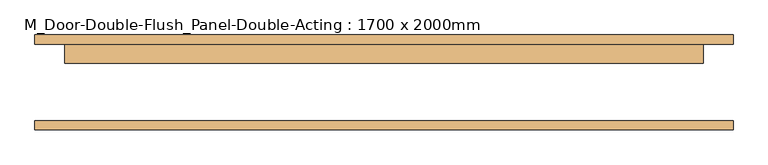
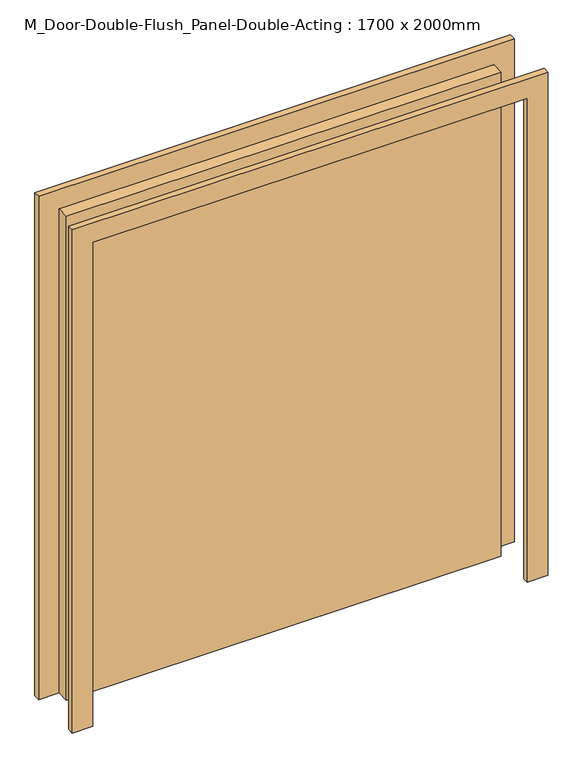
"""IFC4 building model written with IfcOpenShell, lengths in millimetres: door geometry, M_Door-Double-Flush_Panel-Double-Acting : 1700 x 2000mm."""

from ifc_helpers import new_model, si_unit, frame, origin, origin_with_axes, place, context, project, spatial, polyline, outline, extrude, source, transform, mapped, element, save


def m_door_double_flush_panel_double_acting_1700_x_2000mm_ee2ba557(model_context):
    return source(origin(), model_context, "Body", "SweptSolid", [
        extrude(outline(polyline([(2080.0, -930.0), (0.0, -930.0), (0.0, -850.0), (2000.0, -850.0), (2000.0, 850.0), (0.0, 850.0), (0.0, 930.0), (2080.0, 930.0), (2080.0, -930.0)])), frame((0.0, 101.6, 0.0), z_axis=(0.0, 1.0, 0.0), x_axis=(0.0, 0.0, 1.0)), (0.0, 0.0, 1.0), 25.0),
        extrude(outline(polyline([(2000.0, -850.0), (2000.0, 850.0), (0.0, 850.0), (0.0, 930.0), (2080.0, 930.0), (2080.0, -930.0), (0.0, -930.0), (0.0, -850.0), (2000.0, -850.0)])), frame((0.0, -126.6, 0.0), z_axis=(0.0, 1.0, 0.0), x_axis=(0.0, 0.0, 1.0)), (0.0, 0.0, 1.0), 25.0),
        extrude(outline(polyline([(-850.0, 101.6), (850.0, 101.6), (850.0, 51.6), (-850.0, 51.6), (-850.0, 101.6)])), origin_with_axes(), (0.0, 0.0, 1.0), 2000.0),
    ])


if __name__ == "__main__":
    model = new_model("IFC4")
    model_context = context("Model", 3, world=origin())
    ifc_project = project(units=[si_unit("LENGTHUNIT", "METRE", prefix="MILLI")], contexts=[model_context])
    site = spatial("IfcSite", under=ifc_project)
    building = spatial("IfcBuilding", under=site)
    placement = place(None, origin())
    m_door_double_flush_panel_double_acting_1700_x_2000mm_shape = m_door_double_flush_panel_double_acting_1700_x_2000mm_ee2ba557(model_context)
    element("IfcDoor", 1, ObjectType="M_Door-Double-Flush_Panel-Double-Acting : 1700 x 2000mm", at=placement, inside=building, context=model_context, shape_type="MappedRepresentation", body=[
        mapped(m_door_double_flush_panel_double_acting_1700_x_2000mm_shape, transform((0.0, 0.0, 0.0), x_axis=(1.0, 0.0, 0.0), y_axis=(0.0, 1.0, 0.0), z_axis=(0.0, 0.0, 1.0))),
    ])
    save(model, "model.ifc")

# Revit data of these elements
# Type "M_Door-Double-Flush_Panel-Double-Acting : 1700 x 2000mm"
#   Type Mark = "9"
#   Construction Type Id = "DOOR"
#   Assembly Code = "C1020"
#   Analytic Construction = "Wooden"
#   W = 2' - 9.46457"
#   Thickness = 0' - 1.9685"
#   Thermal Resistance (R) = 2.5876 (h·ft²·°F)/BTU
#   Swing Angle [instance default] = 90.00°
#   Heat Transfer Coefficient (U) = 0.3865 BTU/(h·ft²·°F)
#   Height = 6' - 6.74016"
#   Trim Projection Ext. = 0' - 0.98425"
#   Trim Projection Int. = 0' - 0.98425"
#   Trim Width Ext. = 0' - 3.14961"
#   Trim Width Int. = 0' - 3.14961"
#   Width = 5' - 6.92913"
#   Define Thermal Properties by = 1
#   Panel Material = Wood - Birch - Solid Stained Light Low Gloss
#   Trim Material = Paint - Sienna
#   Visual Light Transmittance = 0
#   Solar Heat Gain Coefficient = 0
#   Function = (empty or 0)
#   Wall Closure = (empty or 0)
# Element 1 (IfcDoor, "M_Door-Double-Flush_Panel-Double-Acting : 1700 x 2000mm")
#   Materials on its faces: "Paint - Sienna", "Wood - Birch - Solid Stained Light Low Gloss"
# Materials
#   "Wood - Birch - Solid Stained Light Low Gloss": class "Wood", colour RGB 210 159 95, transparency 0, Cost = 0
#   "Paint - Sienna": colour RGB 118 70 51, transparency 0, Cost = 0
